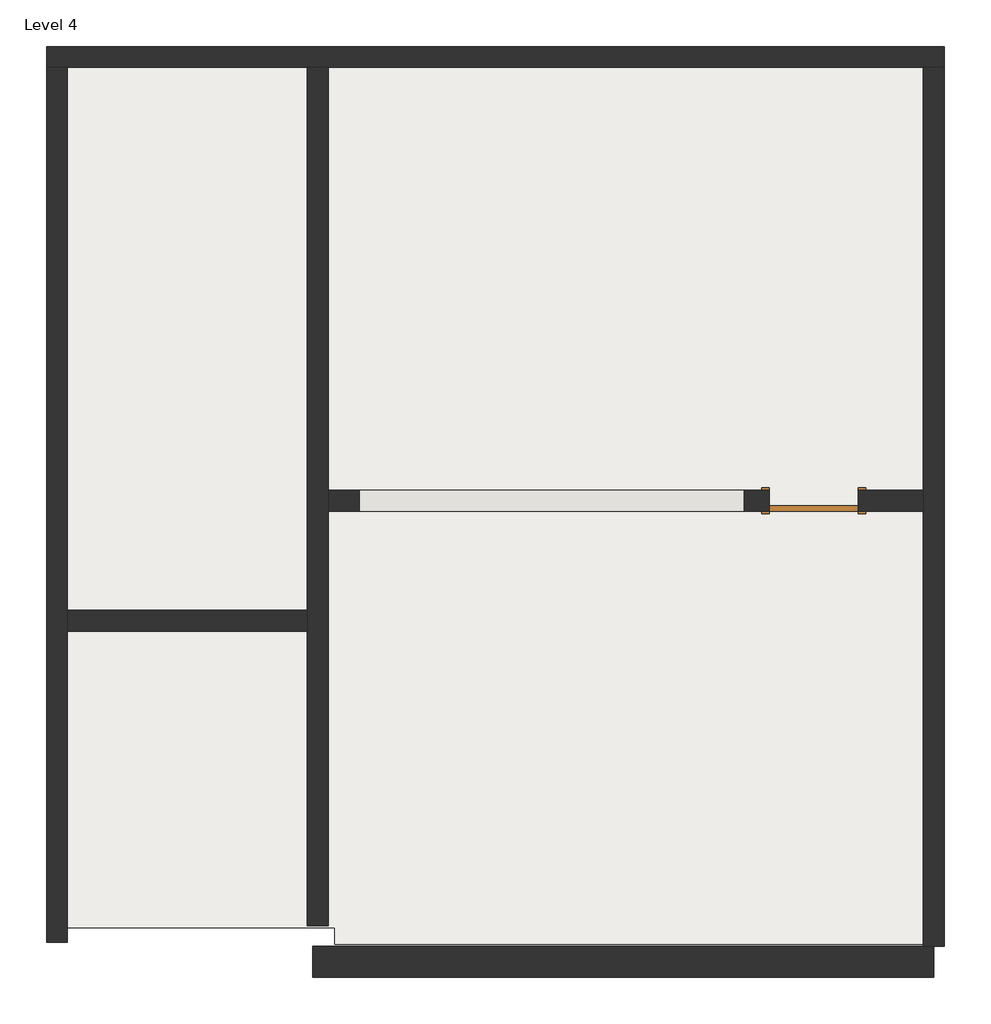
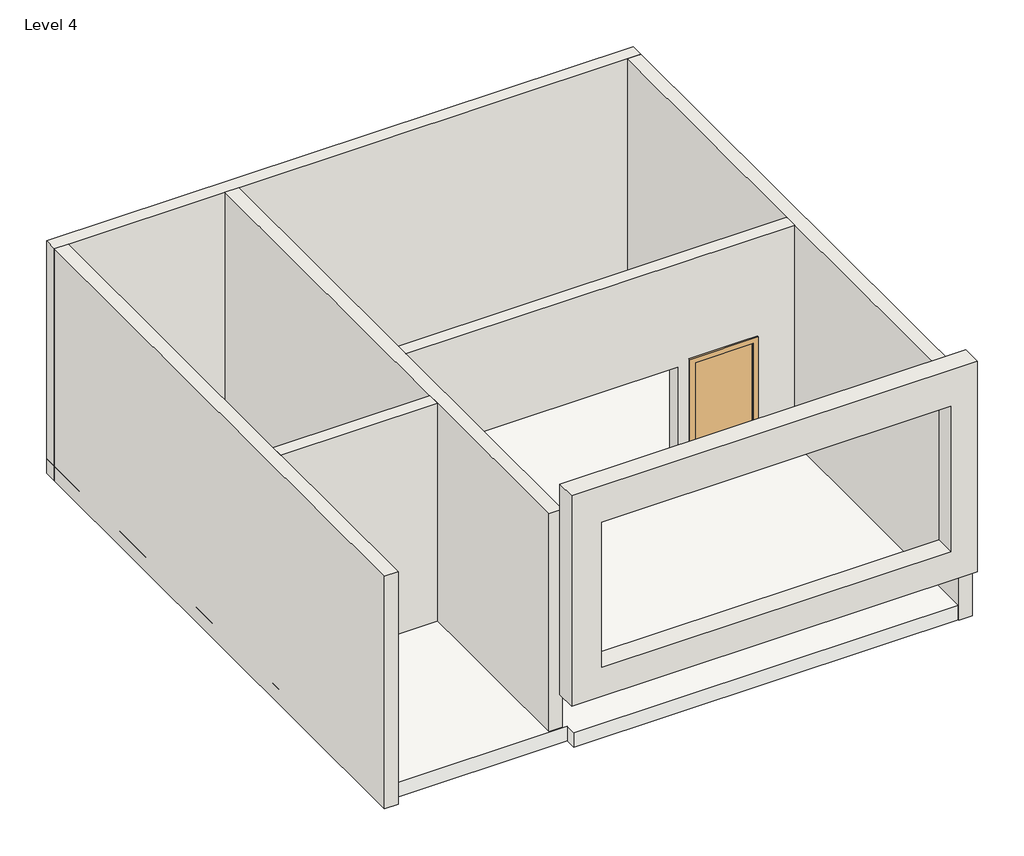
# One storey: 7 walls, 1 door, 1 roof.
"""IFC4 building model written with IfcOpenShell, lengths in millimetres."""

from ifc_helpers import new_model, si_unit, frame, origin, place, context, project, spatial, polyline, outline, extrude, faceted_brep, transform, mapped, element, save
from components import door_10fd3a06, walls_2_walls_1_38dba3ac

model = new_model("IFC4")

# Units and contexts
model_context = context("Model", 3, world=origin())
ifc_project = project(units=[si_unit("LENGTHUNIT", "METRE", prefix="MILLI")], contexts=[model_context])

# Site, building, storey
site = spatial("IfcSite", under=ifc_project)
building = spatial("IfcBuilding", under=site)
storey = spatial("IfcBuildingStorey", under=building, Name="Level 4", Elevation=11887.2)

# Door
placement = place(None, origin())
door_shape = door_10fd3a06(model_context)
element("IfcDoor", 1, ObjectType="Door-Single-Panel : 34\" x 80\"", at=placement, inside=storey, context=model_context, shape_type="MappedRepresentation", body=[
    mapped(door_shape, transform((-1366.3561565, 5783.1985991, 11887.2), x_axis=(-1.0, 0.0, 0.0), y_axis=(0.0, -1.0, 0.0), z_axis=(0.0, 0.0, 1.0))),
])

# Roof
element("IfcRoof", 2, ObjectType="Generic - 9\"", at=placement, inside=storey, context=model_context, shape_type="SweptSolid", body=[
    extrude(outline(polyline([(-8833.9561565, 10202.7985991), (-96.3561565, 10202.7985991), (-96.3561565, 1465.1985991), (-6027.2561565, 1465.1985991), (-6027.2561565, 1623.9485991), (-8833.9561565, 1623.9485991), (-8833.9561565, 10202.7985991)])), frame((0.0, 0.0, 11887.2), z_axis=(0.0, 0.0, 1.0), x_axis=(1.0, 0.0, 0.0)), (0.0, 0.0, 1.0), 228.6),
])

# Walls
element("IfcWall", 3, ObjectType="Generic - 8\"", at=placement, inside=storey, context=model_context, shape_type="SweptSolid", body=[
    extrude(outline(polyline([(-6293.9561565, 4513.1985991), (-8630.7561565, 4513.1985991), (-8630.7561565, 4716.3985991), (-6293.9561565, 4716.3985991), (-6293.9561565, 4513.1985991)])), frame((0.0, 0.0, 11887.2), z_axis=(0.0, 0.0, 1.0), x_axis=(1.0, 0.0, 0.0)), (0.0, 0.0, 1.0), 3657.6),
])
element("IfcWall", 4, ObjectType="Generic - 8\"", at=placement, inside=storey, context=model_context, shape_type="Brep", body=[
    faceted_brep([(-6293.9561565, 9999.5985991, 11887.2), (-6293.9561565, 4716.3985991, 11887.2), (-6293.9561565, 4513.1985991, 11887.2), (-6293.9561565, 1642.9985991, 11887.2), (-6293.9561565, 1642.9985991, 15544.8), (-6293.9561565, 4513.1985991, 15544.8), (-6293.9561565, 4716.3985991, 15544.8), (-6293.9561565, 9999.5985991, 15544.8), (-6090.7561565, 9999.5985991, 11887.2), (-6090.7561565, 9999.5985991, 15544.8), (-6090.7561565, 5884.7985991, 15544.8), (-6090.7561565, 5681.5985991, 15544.8), (-6090.7561565, 1642.9985991, 15544.8), (-6090.7561565, 1642.9985991, 11887.2), (-6090.7561565, 5681.5985991, 11887.2), (-6090.7561565, 5884.7985991, 11887.2)], [[[0, 1, 2, 3, 4, 5, 6, 7]], [[8, 9, 10, 11, 12, 13, 14, 15]], [[3, 2, 1, 0, 8, 15, 14, 13]], [[4, 3, 13, 12]], [[7, 6, 5, 4, 12, 11, 10, 9]], [[0, 7, 9, 8]]]),
])
element("IfcWall", 5, ObjectType="Generic - 8\"", at=placement, inside=storey, context=model_context, shape_type="SweptSolid", body=[
    extrude(outline(polyline([(11887.2, -6090.7561565), (11887.2, -1798.1561565), (13919.2, -1798.1561565), (13919.2, -934.5561565), (11887.2, -934.5561565), (11887.2, -299.5561565), (15544.8, -299.5561565), (15544.8, -6090.7561565), (11887.2, -6090.7561565)]), holes=[polyline([(13913.608423, -2042.3901764), (12152.3392215, -2042.3901764), (12152.3392215, -5792.4012139), (13913.608423, -5792.4012139), (13913.608423, -2042.3901764)])]), frame((0.0, 5681.5985991, 0.0), z_axis=(0.0, 1.0, 0.0), x_axis=(0.0, 0.0, 1.0)), (0.0, 0.0, 1.0), 203.2),
])
element("IfcWall", 6, ObjectType="Generic - 8\"", at=placement, inside=storey, context=model_context, shape_type="Brep", body=[
    faceted_brep([(-8833.9561565, 9999.5985991, 11887.2), (-8630.7561565, 9999.5985991, 11887.2), (-6293.9561565, 9999.5985991, 11887.2), (-6090.7561565, 9999.5985991, 11887.2), (-299.5561565, 9999.5985991, 11887.2), (-96.3561565, 9999.5985991, 11887.2), (-96.3561565, 9999.5985991, 15544.8), (-299.5561565, 9999.5985991, 15544.8), (-6090.7561565, 9999.5985991, 15544.8), (-6293.9561565, 9999.5985991, 15544.8), (-8630.7561565, 9999.5985991, 15544.8), (-8833.9561565, 9999.5985991, 15544.8), (-8833.9561565, 10202.7985991, 11887.2), (-8833.9561565, 10202.7985991, 15544.8), (-96.3561565, 10202.7985991, 15544.8), (-96.3561565, 10202.7985991, 11887.2)], [[[0, 1, 2, 3, 4, 5, 6, 7, 8, 9, 10, 11]], [[12, 13, 14, 15]], [[5, 4, 3, 2, 1, 0, 12, 15]], [[11, 10, 9, 8, 7, 6, 14, 13]], [[6, 5, 15, 14]], [[0, 11, 13, 12]]]),
])
element("IfcWall", 7, ObjectType="Generic - 8\"", at=placement, inside=storey, context=model_context, shape_type="Brep", body=[
    faceted_brep([(-299.5561565, 9999.5985991, 11887.2), (-299.5561565, 5884.7985991, 11887.2), (-299.5561565, 5681.5985991, 11887.2), (-299.5561565, 1446.1485991, 11887.2), (-299.5561565, 1446.1485991, 11891.0745283), (-299.5561565, 1446.1485991, 13131.8), (-299.5561565, 1446.1485991, 15544.8), (-299.5561565, 1465.1985991, 15544.8), (-299.5561565, 5681.5985991, 15544.8), (-299.5561565, 5884.7985991, 15544.8), (-299.5561565, 9999.5985991, 15544.8), (-96.3561565, 9999.5985991, 11887.2), (-96.3561565, 9999.5985991, 15544.8), (-96.3561565, 1465.1985991, 15544.8), (-96.3561565, 1446.1485991, 15544.8), (-96.3561565, 1446.1485991, 11887.2)], [[[0, 1, 2, 3, 4, 5, 6, 7, 8, 9, 10]], [[11, 12, 13, 14, 15]], [[3, 2, 1, 0, 11, 15]], [[7, 6, 14, 13]], [[10, 9, 8, 7, 13, 12]], [[6, 5, 4, 3, 15, 14]], [[0, 10, 12, 11]]]),
])
element("IfcWall", 8, ObjectType="Generic - 8\"", at=placement, inside=storey, context=model_context, shape_type="Brep", body=[
    faceted_brep([(-8630.7561565, 1484.2485991, 11887.2), (-8630.7561565, 4513.1985991, 11887.2), (-8630.7561565, 4716.3985991, 11887.2), (-8630.7561565, 9999.5985991, 11887.2), (-8630.7561565, 9999.5985991, 15544.8), (-8630.7561565, 4716.3985991, 15544.8), (-8630.7561565, 4513.1985991, 15544.8), (-8630.7561565, 1484.2485991, 15544.8), (-8833.9561565, 1484.2485991, 11887.2), (-8833.9561565, 1484.2485991, 15544.8), (-8833.9561565, 9999.5985991, 15544.8), (-8833.9561565, 9999.5985991, 11887.2)], [[[0, 1, 2, 3, 4, 5, 6, 7]], [[8, 9, 10, 11]], [[3, 2, 1, 0, 8, 11]], [[7, 6, 5, 4, 10, 9]], [[0, 7, 9, 8]], [[4, 3, 11, 10]]]),
])
walls_2_walls_1_shape = walls_2_walls_1_38dba3ac(model_context)
element("IfcWall", 9, ObjectType="Walls 2 : Walls 1", at=placement, inside=storey, context=model_context, shape_type="MappedRepresentation", body=[
    mapped(walls_2_walls_1_shape, transform((0.0, 0.0, 0.0), x_axis=(1.0, 0.0, 0.0), y_axis=(0.0, 1.0, 0.0), z_axis=(0.0, 0.0, 1.0))),
])

save(model, "model.ifc")

# Revit data of these elements
# Type "Door-Single-Panel : 34\" x 80\""
#   Type Mark = "8"
#   Construction Type Id = "DOOR"
#   Assembly Code = "C1020300"
#   Analytic Construction = "Wooden"
#   Thickness = 0' - 2"
#   Thermal Resistance (R) = 2.5876 (h·ft²·°F)/BTU
#   Swing Angle [instance default] = 90.00°
#   Heat Transfer Coefficient (U) = 0.3865 BTU/(h·ft²·°F)
#   Height = 6' - 8"
#   Trim Projection Ext = 0' - 1"
#   Trim Projection Int = 0' - 1"
#   Trim Width = 0' - 3"
#   Width = 2' - 10"
#   Define Thermal Properties by = 1
#   Panel Material = Wood - Birch - Solid Stained Light Low Gloss
#   Trim Material = Paint - Sienna
#   Visual Light Transmittance = 0
#   Solar Heat Gain Coefficient = 0
#   Function = (empty or 0)
#   Wall Closure = (empty or 0)
# Type "Generic - 9\""
#   Assembly Code = "B1020"
#   Layers, outside or top first: 0' - 9" no material (function 1)
# Type "Generic - 8\""
#   Assembly Code = "B2010"
#   Layers, outside or top first: 0' - 8" no material (function 1)
# Element 1 (IfcDoor, "Door-Single-Panel : 34\" x 80\"")
#   Swing Angle = 90.00°
#   Phase Created = New Construction
#   Materials on its faces: "Paint - Sienna", "Wood - Birch - Solid Stained Light Low Gloss"
# Element 2 (IfcRoof, "Generic - 9\"")
#   built-in parameter 1001705 = 39.75 (stored number, unit not read)
#   built-in parameter 1001710 = 33615
#   Phase Created = New Construction
#   Materials on its faces: "Default Roof"
# Elements 3, 4, 5, 6, 7, 8 (IfcWall, "Generic - 8\"")
#   Top Offset = 0' - 0"
#   Base Offset = 0' - 0"
#   Unconnected Height = 12' - 0"
#   wall height = 12' - 0"
#   Phase Created = New Construction
#   Base Constraint = Level 4
#   Materials on its faces: "Default Wall"
# Element 9 (IfcWall, "Walls 2 : Walls 1")
#   Phase Created = New Construction
#   Materials on its faces: "Default Wall"
# Materials
#   "Wood - Birch - Solid Stained Light Low Gloss": class "Wood", colour RGB 210 159 95, transparency 0, Cost = 0
#   "Paint - Sienna": colour RGB 118 70 51, transparency 0, Cost = 0
#   "Default Roof": colour RGB 88 101 114, transparency 0
#   "Default Wall": colour RGB 128 128 128, transparency 0
